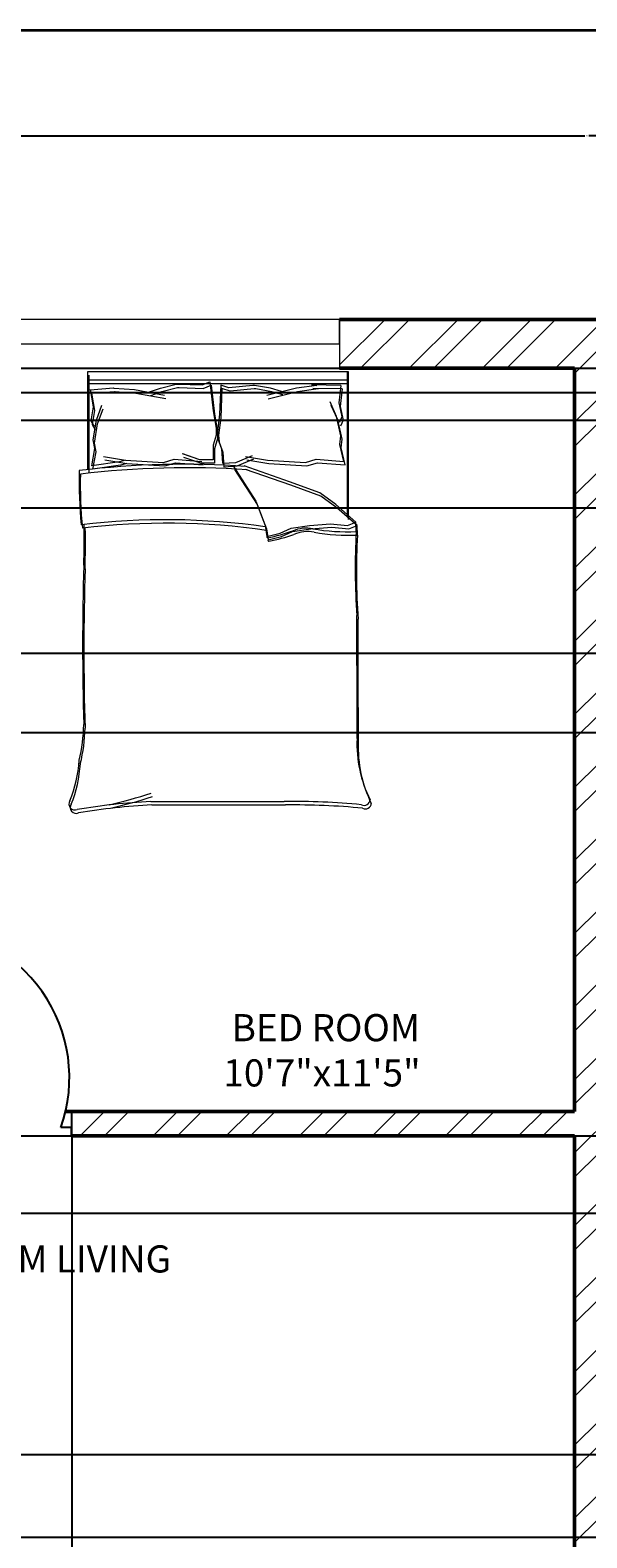
# Model space of a CAD drawing. Units: inches. Extents: x 2310 to 2937, y 1113 to 2410.
# Tile 19 of 23: x 2507 to 2609, y 2132 to 2410. Entities that reach past the tile are written whole.
import ezdxf

# ---------------------------------------------------------------- set-up
doc = ezdxf.new("R2010")
doc.units = ezdxf.units.IN
for name, color, linetype, lineweight in [('A-ANNO-DIMS', 2, 'Continuous', 18), ('A-ANNO-TTLB', 7, 'Continuous', 35), ('A-AREA-IDEN', 7, 'Continuous', 18), ('A-DOOR', 31, 'Continuous', 25), ('A-FURN', 8, 'Continuous', 18), ('A-GLAZ', 191, 'Continuous', 20), ('A-WALL', 7, 'Continuous', 50), ('A-WALL-PATT', 85, 'Continuous', 13)]:
    doc.layers.add(name, color=color, linetype=linetype, lineweight=lineweight)
doc.styles.get("Standard").update_dxf_attribs({"font": 'arial.ttf'})
doc.dimstyles.get("Standard").update_dxf_attribs({"dimtxt": 0.18, "dimasz": 0.18, "dimexe": 0.18, "dimexo": 0.0625, "dimgap": 0.09, "dimtad": 0, "dimtih": 1, "dimtoh": 1, "dimdec": 4, "dimzin": 0, "dimdsep": 46, "dimtxsty": 'Standard', "dimcen": 0.09, "dimadec": 0, "dimazin": 0, "dimtfac": 1, "dimtdec": 4, "dimtofl": 0, "dimtmove": 0, "dimatfit": 3, "dimfxl": 1, "dimtolj": 1, "dimtzin": 0, "dimarcsym": 0})

# ---------------------------------------------------------------- blocks, each defined once
blk = doc.blocks.new('BED-DOUBLE')
for p, q in [((3.56, 63.44), (3.56, 81.55)), ((3.56, 63.44), (3.56, 81.55)), ((3.56, 81.55), (51.58, 81.55)), ((3.79, 62.8), (3.79, 80.91)), ((3.79, 62.8), (3.79, 80.91)), ((51.35, 81.55), (51.35, 54.94)), ((51.35, 81.55), (51.35, 54.94)), ((51.58, 81.55), (51.58, 80.91)), ((51.58, 80.91), (51.58, 54.3)), ((51.58, 80.91), (51.58, 54.3)), ((3.56, 80.01), (51.35, 80.01)), ((3.56, 80.01), (51.35, 80.01)), ((3.79, 79.38), (51.58, 79.38)), ((3.79, 79.38), (51.58, 79.38)), ((3.98, 78.21), (8.27, 78.54)), ((3.98, 78.23), (4.56, 75.05)), ((3.98, 78.23), (4.56, 75.05)), ((3.99, 78.21), (8.27, 78.54)), ((4.21, 77.57), (8.49, 77.9)), ((4.21, 77.57), (8.49, 77.9)), ((8.27, 78.54), (8.37, 78.52)), ((8.27, 78.54), (8.37, 78.52)), ((8.37, 78.52), (12.19, 78.23)), ((8.37, 78.52), (12.19, 78.23)), ((8.49, 77.9), (8.6, 77.88)), ((8.49, 77.9), (8.6, 77.88)), ((8.6, 77.88), (12.42, 77.59)), ((8.6, 77.88), (12.42, 77.59)), ((12.19, 78.23), (17.69, 77.22)), ((12.19, 78.23), (17.69, 77.22)), ((14.94, 77.8), (16.97, 78.52)), ((14.94, 77.8), (16.96, 78.52)), ((15.17, 77.16), (17.19, 77.88)), ((15.17, 77.16), (17.19, 77.88)), ((16.96, 78.52), (19.86, 79.24)), ((16.97, 78.52), (19.86, 79.24)), ((17.19, 77.88), (20.08, 78.61)), ((17.19, 77.88), (20.08, 78.61)), ((19.86, 79.24), (20.18, 79.24)), ((19.86, 79.24), (20.18, 79.24)), ((20.08, 78.61), (20.41, 78.61)), ((20.08, 78.61), (20.41, 78.61)), ((20.18, 79.24), (24.62, 79.1)), ((20.18, 79.24), (24.62, 79.1)), ((20.41, 78.61), (24.85, 78.46)), ((20.41, 78.61), (24.85, 78.46)), ((24.62, 79.1), (26.07, 79.68)), ((24.62, 79.1), (26.07, 79.68)), ((24.85, 78.46), (26.3, 79.04)), ((24.85, 78.46), (26.3, 79.04)), ((26.07, 79.68), (26.65, 74.33)), ((26.07, 79.68), (26.65, 74.33)), ((26.3, 79.04), (26.88, 73.69)), ((26.3, 79.04), (26.88, 73.69)), ((28.06, 79.06), (27.82, 73.68)), ((28.06, 79.06), (27.82, 73.68)), ((28.29, 78.42), (28.05, 73.04)), ((28.29, 78.42), (28.05, 73.04)), ((29.54, 78.57), (28.06, 79.06)), ((29.54, 78.57), (28.06, 79.06)), ((29.77, 77.93), (28.29, 78.42)), ((29.77, 77.93), (28.29, 78.42)), ((33.97, 78.99), (29.54, 78.57)), ((33.97, 78.99), (29.54, 78.57)), ((34.2, 78.35), (29.77, 77.93)), ((34.2, 78.35), (29.77, 77.93)), ((34.29, 79.01), (33.97, 78.99)), ((34.29, 79.01), (33.97, 78.99)), ((34.52, 78.37), (34.2, 78.35)), ((34.52, 78.37), (34.2, 78.35)), ((37.22, 78.47), (34.29, 79.01)), ((37.22, 78.47), (34.29, 79.01)), ((37.45, 77.83), (34.52, 78.37)), ((37.45, 77.83), (34.52, 78.37)), ((42, 78.48), (36.58, 77.13)), ((42, 78.48), (36.58, 77.13)), ((42.23, 77.84), (36.81, 76.49)), ((42.23, 77.84), (36.81, 76.49)), ((39.29, 77.87), (37.22, 78.47)), ((39.29, 77.87), (37.22, 78.47)), ((39.52, 77.24), (37.45, 77.83)), ((39.51, 77.24), (37.45, 77.83)), ((45.8, 79.01), (42, 78.48)), ((45.8, 79.01), (42, 78.48)), ((46.03, 78.37), (42.23, 77.84)), ((46.03, 78.37), (42.23, 77.84)), ((50.2, 78.99), (44.8, 79.09)), ((44.8, 79.09), (45.8, 79.01)), ((50.2, 78.99), (44.8, 79.09)), ((44.8, 79.09), (45.8, 79.01)), ((50.43, 78.35), (45.02, 78.45)), ((45.02, 78.45), (46.03, 78.37)), ((50.43, 78.35), (45.02, 78.45)), ((45.02, 78.45), (46.03, 78.37)), ((50.2, 78.99), (49.82, 75.78)), ((50.2, 78.99), (49.82, 75.78)), ((50.43, 78.35), (50.05, 75.14)), ((50.43, 78.35), (50.05, 75.14)), ((4.56, 75.05), (4.13, 72.45)), ((4.56, 75.05), (4.13, 72.45)), ((4.21, 77.59), (4.79, 74.41)), ((4.21, 77.59), (4.79, 74.41)), ((5.14, 72.59), (6.15, 75.34)), ((5.14, 72.59), (6.15, 75.34)), ((12.42, 77.59), (17.92, 76.58)), ((12.42, 77.59), (17.92, 76.58)), ((49.4, 73.29), (48.21, 75.97)), ((49.4, 73.29), (48.21, 75.97)), ((49.62, 72.65), (48.44, 75.33)), ((49.62, 72.65), (48.44, 75.33)), ((49.82, 75.78), (50.42, 73.21)), ((49.82, 75.78), (50.41, 73.21)), ((50.05, 75.14), (50.64, 72.57)), ((50.05, 75.14), (50.64, 72.57)), ((4.13, 72.45), (4.7, 71.44)), ((4.13, 72.45), (4.7, 71.44)), ((4.79, 74.41), (4.35, 71.81)), ((4.79, 74.41), (4.35, 71.81)), ((4.56, 68.98), (5.14, 72.59)), ((4.56, 68.98), (5.14, 72.59)), ((5.37, 71.95), (6.38, 74.7)), ((5.37, 71.95), (6.38, 74.7)), ((26.65, 74.33), (27.23, 71.15)), ((26.65, 74.33), (27.23, 71.15)), ((26.88, 73.69), (27.45, 70.51)), ((26.88, 73.69), (27.45, 70.51)), ((27.82, 73.68), (27.44, 70.47)), ((27.82, 73.68), (27.44, 70.47)), ((28.05, 73.04), (27.67, 69.83)), ((28.05, 73.04), (27.67, 69.83)), ((50.2, 69.72), (49.4, 73.29)), ((50.2, 69.72), (49.4, 73.29)), ((50.43, 69.08), (49.62, 72.65)), ((50.43, 69.08), (49.62, 72.65)), ((50.42, 73.21), (49.9, 72.16)), ((50.41, 73.21), (49.9, 72.16)), ((50.64, 72.57), (50.13, 71.52)), ((50.64, 72.57), (50.13, 71.52)), ((4.35, 71.81), (4.93, 70.8)), ((4.35, 71.81), (4.93, 70.8)), ((4.79, 68.34), (5.37, 71.95)), ((4.79, 68.34), (5.37, 71.95)), ((27.23, 69.85), (26.65, 67.97)), ((27.23, 69.85), (26.65, 67.97)), ((27.23, 71.15), (27.23, 69.85)), ((27.23, 71.15), (27.23, 69.85)), ((27.44, 70.47), (27.52, 69.17)), ((27.44, 70.47), (27.52, 69.17)), ((27.45, 70.51), (27.45, 69.21)), ((27.45, 70.51), (27.45, 69.21)), ((27.67, 69.83), (27.75, 68.53)), ((27.67, 69.83), (27.75, 68.53)), ((50.01, 68.11), (50.2, 69.72)), ((50.01, 68.11), (50.2, 69.72)), ((4.27, 64.21), (4.85, 67.39)), ((4.27, 64.21), (4.85, 67.39)), ((4.5, 63.57), (5.08, 66.75)), ((4.5, 63.57), (5.08, 66.75)), ((4.85, 67.39), (4.56, 68.98)), ((4.85, 67.39), (4.56, 68.98)), ((5.08, 66.75), (4.79, 68.34)), ((5.08, 66.75), (4.79, 68.34)), ((26.65, 67.97), (26.65, 65.29)), ((26.65, 67.97), (26.65, 65.29)), ((27.45, 69.21), (26.88, 67.33)), ((27.45, 69.21), (26.88, 67.33)), ((26.88, 67.33), (26.88, 64.65)), ((26.88, 67.33), (26.88, 64.65)), ((27.52, 69.17), (28.22, 67.33)), ((27.52, 69.17), (28.22, 67.33)), ((27.75, 68.53), (28.45, 66.69)), ((27.75, 68.53), (28.44, 66.69)), ((28.22, 67.33), (28.38, 64.66)), ((28.22, 67.33), (28.38, 64.66)), ((50.78, 64.98), (50.01, 68.11)), ((50.78, 64.98), (50.01, 68.11)), ((50.24, 67.48), (50.43, 69.08)), ((50.24, 67.48), (50.43, 69.08)), ((51.01, 64.34), (50.24, 67.48)), ((51.01, 64.34), (50.24, 67.48)), ((9.37, 64.93), (4.27, 64.21)), ((9.37, 64.93), (4.27, 64.21)), ((9.6, 64.29), (4.5, 63.57)), ((9.6, 64.29), (4.5, 63.57)), ((6.47, 65.92), (10.5, 65.25)), ((6.47, 65.92), (10.5, 65.25)), ((6.7, 65.28), (10.73, 64.61)), ((6.7, 65.28), (10.73, 64.61)), ((10.5, 65.25), (9.37, 64.93)), ((10.5, 65.25), (9.37, 64.93)), ((10.73, 64.61), (9.6, 64.29)), ((10.73, 64.61), (9.6, 64.29)), ((10.5, 65.25), (17.51, 64.82)), ((10.5, 65.25), (17.51, 64.82)), ((10.73, 64.61), (17.74, 64.18)), ((10.73, 64.61), (17.74, 64.18)), ((17.51, 64.82), (19.47, 65.38)), ((17.51, 64.82), (19.47, 65.38)), ((17.74, 64.18), (19.7, 64.74)), ((17.74, 64.18), (19.7, 64.74)), ((19.47, 65.38), (24.6, 64.98)), ((19.47, 65.38), (24.6, 64.98)), ((19.7, 64.74), (24.83, 64.34)), ((19.7, 64.74), (24.83, 64.34)), ((24.19, 65.29), (21.04, 66.38)), ((24.19, 65.29), (21.05, 66.38)), ((24.42, 64.65), (21.27, 65.74)), ((24.42, 64.65), (21.27, 65.74)), ((26.65, 65.29), (24.19, 65.29)), ((26.65, 65.29), (24.19, 65.29)), ((26.88, 64.65), (24.42, 64.65)), ((26.88, 64.65), (24.42, 64.65)), ((28.38, 64.66), (30.84, 64.81)), ((28.38, 64.66), (30.84, 64.81)), ((28.44, 66.69), (28.61, 64.02)), ((28.45, 66.69), (28.61, 64.02)), ((28.61, 64.02), (31.07, 64.17)), ((28.61, 64.02), (31.06, 64.17)), ((30.35, 64.17), (34.54, 57.67)), ((30.35, 64.17), (34.54, 57.67)), ((30.84, 64.81), (33.91, 66.09)), ((30.84, 64.81), (33.91, 66.09)), ((31.06, 64.17), (34.14, 65.45)), ((31.07, 64.17), (34.14, 65.45)), ((40.73, 61.23), (32.39, 64.17)), ((40.73, 61.23), (32.39, 64.17)), ((32.65, 65.92), (36.68, 65.25)), ((32.65, 65.92), (36.68, 65.25)), ((32.88, 65.28), (36.91, 64.61)), ((32.88, 65.28), (36.91, 64.61)), ((36.68, 65.25), (43.69, 64.82)), ((36.68, 65.25), (43.69, 64.82)), ((36.91, 64.61), (43.92, 64.18)), ((36.91, 64.61), (43.92, 64.18)), ((43.69, 64.82), (45.65, 65.38)), ((43.69, 64.82), (45.65, 65.38)), ((43.92, 64.18), (45.88, 64.74)), ((43.92, 64.18), (45.88, 64.74)), ((45.65, 65.38), (50.78, 64.98)), ((45.65, 65.38), (50.78, 64.98)), ((45.88, 64.74), (51.01, 64.34)), ((45.88, 64.74), (51.01, 64.34)), ((30.57, 63.53), (34.76, 57.03)), ((30.57, 63.53), (34.76, 57.03)), ((40.96, 60.59), (32.62, 63.53)), ((40.96, 60.59), (32.62, 63.53)), ((46.31, 59.22), (40.73, 61.23)), ((46.31, 59.22), (40.73, 61.23)), ((46.53, 58.58), (40.96, 60.59)), ((46.53, 58.58), (40.96, 60.59)), ((49.25, 57.05), (46.31, 59.22)), ((49.25, 57.05), (46.31, 59.22)), ((49.48, 56.41), (46.53, 58.58)), ((49.48, 56.41), (46.53, 58.58)), ((34.54, 57.67), (36.24, 53.18)), ((34.54, 57.67), (36.24, 53.18)), ((34.76, 57.03), (36.47, 52.54)), ((34.76, 57.03), (36.47, 52.54)), ((52.95, 53.8), (49.25, 57.05)), ((52.95, 53.8), (49.25, 57.05)), ((53.18, 53.16), (49.48, 56.41)), ((53.18, 53.16), (49.48, 56.41)), ((36.24, 53.18), (36.55, 51.17)), ((36.24, 53.18), (36.55, 51.17)), ((41.04, 52.72), (44.45, 53.18)), ((41.04, 52.72), (44.45, 53.18)), ((44.45, 53.18), (48.32, 53.49)), ((44.45, 53.18), (48.32, 53.49)), ((44.68, 52.54), (48.55, 52.85)), ((44.68, 52.54), (48.55, 52.85)), ((48.32, 53.49), (51.42, 53.18)), ((48.32, 53.49), (51.42, 53.18)), ((48.55, 52.85), (51.65, 52.54)), ((48.55, 52.85), (51.65, 52.54)), ((51.42, 53.18), (52.95, 53.8)), ((51.42, 53.18), (52.95, 53.8)), ((51.65, 52.54), (53.18, 53.16)), ((51.65, 52.54), (53.18, 53.16)), ((53.03, 52.06), (52.95, 53.8, 3.87)), ((53.03, 52.06), (52.95, 53.8, 3.87)), ((53.26, 51.42), (53.18, 53.16, 3.87)), ((53.26, 51.42), (53.18, 53.16, 3.87)), ((36.47, 52.54), (36.78, 50.53)), ((36.47, 52.54), (36.78, 50.53)), ((36.55, 51.17), (39.03, 51.79)), ((36.55, 51.17), (39.03, 51.79)), ((36.78, 50.53), (39.26, 51.15)), ((36.78, 50.53), (39.26, 51.15)), ((39.03, 51.79), (41.04, 52.72)), ((39.03, 51.79), (41.04, 52.72)), ((39.26, 51.15), (41.27, 52.08)), ((39.26, 51.15), (41.27, 52.08)), ((41.27, 52.08), (44.68, 52.54)), ((41.27, 52.08), (44.68, 52.54)), ((15.15, 2.3), (39.76, 2.3)), ((15.15, 2.3), (39.76, 2.3)), ((15.38, 1.66), (39.99, 1.66)), ((15.38, 1.66), (39.99, 1.66))]:
    blk.add_line(p, q)
for centre, radius, start, end in [((21.45, -100.5), 164.97, 86.0865, 96.7821), ((21.45, -100.5), 164.97, 86.0865, 96.7821), ((85.25, 61.45), 83.31, 178.7218, 185.604), ((85.25, 61.45), 83.31, 178.7218, 185.604), ((85.48, 60.81), 83.31, 178.7218, 185.604), ((85.48, 60.81), 83.31, 178.7218, 185.604), ((21.67, -101.14), 164.97, 86.0865, 96.7821), ((21.67, -101.14), 164.97, 86.0865, 96.7821), ((17.84, -74.77), 129.02, 81.7845, 96.9006), ((17.84, -74.77), 129.02, 81.7845, 96.9006), ((18.07, -75.41), 129.02, 81.7845, 96.9006), ((18.07, -75.41), 129.02, 81.7845, 96.9006), ((-167.22, 50.37), 170.11, 358.4762, 1.0082), ((-167.22, 50.37), 170.11, 358.4762, 1.0082), ((-166.99, 49.74), 170.11, 358.4762, 1.0082), ((-166.99, 49.74), 170.11, 358.4762, 1.0082), ((36.72, 51.11), 0.185, 160.2464, 271.1377), ((36.72, 51.11), 0.185, 160.2464, 271.1377), ((31.24, 80.07), 29.65, 280.6617, 289.8806), ((31.24, 80.07), 29.65, 280.6617, 289.8806), ((36.95, 50.47), 0.185, 160.2464, 271.1377), ((36.95, 50.47), 0.185, 160.2464, 271.1377), ((31.47, 79.43), 29.65, 280.6617, 289.8806), ((31.47, 79.43), 29.65, 280.6617, 289.8806), ((43.83, 46.48), 6.22, 78.6608, 113.7384), ((43.83, 46.48), 6.22, 78.6608, 113.7384), ((44.06, 45.84), 6.22, 78.6608, 113.7384), ((44.06, 45.84), 6.22, 78.6608, 113.7384), ((51.41, 88.2), 36.18, 259.8763, 272.5657), ((51.41, 88.2), 36.18, 259.8763, 272.5657), ((51.64, 87.57), 36.18, 259.8763, 272.5657), ((51.64, 87.57), 36.18, 259.8763, 272.5657), ((182.35, 45.23), 129.5, 176.9791, 183.8365), ((182.35, 45.23), 129.5, 176.9791, 183.8365), ((182.58, 44.59), 129.5, 176.9791, 183.8365), ((182.58, 44.59), 129.5, 176.9791, 183.8365), ((484.91, 30.93), 482.31, 178.2277, 181.7185), ((484.91, 30.93), 482.31, 178.2277, 181.7185), ((485.14, 30.3), 482.31, 178.2277, 181.7185), ((485.14, 30.3), 482.31, 178.2277, 181.7185), ((-4508.66, 13.73), 4561.86, 0.00217, 0.28689), ((-4508.66, 13.73), 4561.86, 0.00217, 0.28689), ((-4508.43, 13.09), 4561.86, 0.00217, 0.28689), ((-4508.43, 13.09), 4561.86, 0.00217, 0.28689), ((-26.81, 17.03), 29.63, 346.0648, 358.9113), ((-26.81, 17.03), 29.63, 346.0648, 358.9113), ((-26.58, 16.39), 29.63, 346.0648, 358.9113), ((-26.58, 16.39), 29.63, 346.0648, 358.9113), ((76.24, 12.88), 23.07, 177.4714, 206.4681), ((76.24, 12.88), 23.07, 177.4714, 206.4681), ((76.47, 12.24), 23.07, 177.4714, 206.4681), ((76.47, 12.24), 23.07, 177.4714, 206.4681), ((-21.57, 11.27), 23.56, 337.9751, 356.652), ((-21.57, 11.27), 23.56, 337.9751, 356.652), ((-21.34, 10.63), 23.56, 337.9751, 356.652), ((-21.34, 10.63), 23.56, 337.9751, 356.652), ((-17.14, 105.26), 106.46, 283.3832, 287.7053), ((-17.14, 105.26), 106.46, 283.3832, 287.7053), ((-16.91, 104.62), 106.46, 283.3832, 287.7053), ((-16.91, 104.62), 106.46, 283.3832, 287.7053), ((1.17, 1.83), 1.09, 146.1736, 293.4781), ((1.17, 1.83), 1.09, 146.1736, 293.4781), ((1.4, 1.19), 1.09, 146.1736, 293.4781), ((1.4, 1.19), 1.09, 146.1736, 293.4781), ((21.51, -119.29), 121.76, 92.9958, 99.4091), ((21.51, -119.29), 121.76, 92.9958, 99.4091), ((21.74, -119.93), 121.76, 92.9958, 99.4091), ((21.74, -119.93), 121.76, 92.9958, 99.4091), ((41.24, -130.73), 133.04, 84.4998, 90.6351), ((41.24, -130.73), 133.04, 84.4998, 90.6351), ((41.47, -131.37), 133.04, 84.4998, 90.6351), ((41.47, -131.37), 133.04, 84.4998, 90.6351), ((54.5, 2.68), 1.1, 242.6588, 356.02), ((54.5, 2.68), 1.1, 242.6588, 356.02), ((54.72, 2.04), 1.1, 242.6588, 356.02), ((54.72, 2.04), 1.1, 242.6588, 356.02)]:
    blk.add_arc(centre, radius, start, end)
blk = doc.blocks.new('WIN-60IN-HEAD')
for p, q in [((0, 0), (0, 9)), ((0, 9), (0, 4.5)), ((60, 9), (0, 9)), ((60, 4.5), (60, 9)), ((60, 9), (60, 0)), ((0, 4.5), (60, 4.5)), ((0, 0), (60, 0))]:
    blk.add_line(p, q)
blk = doc.blocks.new('*D39')
at = {"layer": 'A-ANNO-DIMS', "color": 0, "lineweight": -2, "transparency": 16777216}
for p, q in [((2394.49, 2356.58), (2394.49, 2390.54)), ((2394.67, 2390.36), (2608.84, 2390.36)), ((2823.81, 2390.36), (2609.63, 2390.36)), ((2823.99, 2356.58), (2823.99, 2390.54))]:
    blk.add_line(p, q, dxfattribs=at)
at = {"layer": 'A-ANNO-DIMS', "color": 0, "transparency": 16777216}
for points in [[(2394.67, 2390.39), (2394.67, 2390.33), (2394.49, 2390.36)], [(2823.81, 2390.39), (2823.81, 2390.33), (2823.99, 2390.36)]]:
    blk.add_solid(points, dxfattribs=at)
at = {"layer": 'Defpoints', "color": 0, "transparency": 16777216}
for p in [(2823.99, 2390.36), (2394.49, 2356.51), (2823.99, 2356.51)]:
    blk.add_point(p, dxfattribs=at)
at = {"layer": 'A-ANNO-DIMS', "color": 0, "transparency": 16777216, "insert": (2609.24, 2390.36), "char_height": 0.18, "attachment_point": 5}
blk.add_mtext('\\A1;429.5', dxfattribs=at)
blk = doc.blocks.new('*D52')
at = {"layer": 'A-ANNO-DIMS', "color": 0, "lineweight": -2, "transparency": 16777216}
for p, q in [((2403.55, 2347.51), (2858.02, 2347.51)), ((2857.84, 2347.33), (2857.84, 2342.9)), ((2857.84, 2338.1), (2857.84, 2342.54)), ((2403.55, 2337.92), (2858.02, 2337.92))]:
    blk.add_line(p, q, dxfattribs=at)
at = {"layer": 'A-ANNO-DIMS', "color": 0, "transparency": 16777216}
for points in [[(2857.81, 2347.33), (2857.87, 2347.33), (2857.84, 2347.51)], [(2857.81, 2338.1), (2857.87, 2338.1), (2857.84, 2337.92)]]:
    blk.add_solid(points, dxfattribs=at)
at = {"layer": 'Defpoints', "color": 0, "transparency": 16777216}
for p in [(2403.49, 2347.51), (2403.49, 2337.92), (2857.84, 2337.92)]:
    blk.add_point(p, dxfattribs=at)
at = {"layer": 'A-ANNO-DIMS', "color": 0, "transparency": 16777216, "insert": (2857.84, 2342.72), "char_height": 0.18, "attachment_point": 5}
blk.add_mtext('\\A1;9.59', dxfattribs=at)
blk = doc.blocks.new('*D53')
at = {"layer": 'A-ANNO-DIMS', "color": 0, "lineweight": -2, "transparency": 16777216}
for p, q in [((2403.55, 2295.01), (2858.02, 2295.01)), ((2857.84, 2294.83), (2857.84, 2287.87)), ((2857.84, 2280.55), (2857.84, 2287.51)), ((2403.55, 2280.37), (2858.02, 2280.37))]:
    blk.add_line(p, q, dxfattribs=at)
at = {"layer": 'A-ANNO-DIMS', "color": 0, "transparency": 16777216}
for points in [[(2857.81, 2294.83), (2857.87, 2294.83), (2857.84, 2295.01)], [(2857.81, 2280.55), (2857.87, 2280.55), (2857.84, 2280.37)]]:
    blk.add_solid(points, dxfattribs=at)
at = {"layer": 'Defpoints', "color": 0, "transparency": 16777216}
for p in [(2403.49, 2295.01), (2403.49, 2280.37), (2857.84, 2280.37)]:
    blk.add_point(p, dxfattribs=at)
at = {"layer": 'A-ANNO-DIMS', "color": 0, "transparency": 16777216, "insert": (2857.84, 2287.69), "char_height": 0.18, "attachment_point": 5}
blk.add_mtext('\\A1;14.644', dxfattribs=at)
blk = doc.blocks.new('*D54')
at = {"layer": 'A-ANNO-DIMS', "color": 0, "lineweight": -2, "transparency": 16777216}
for p, q in [((2403.55, 2206.01), (2858.02, 2206.01)), ((2857.84, 2205.83), (2857.84, 2199.07)), ((2857.84, 2191.94), (2857.84, 2198.7)), ((2403.55, 2191.76), (2858.02, 2191.76))]:
    blk.add_line(p, q, dxfattribs=at)
at = {"layer": 'A-ANNO-DIMS', "color": 0, "transparency": 16777216}
for points in [[(2857.81, 2205.83), (2857.87, 2205.83), (2857.84, 2206.01)], [(2857.81, 2191.94), (2857.87, 2191.94), (2857.84, 2191.76)]]:
    blk.add_solid(points, dxfattribs=at)
at = {"layer": 'Defpoints', "color": 0, "transparency": 16777216}
for p in [(2403.49, 2206.01), (2403.49, 2191.76), (2857.84, 2191.76)]:
    blk.add_point(p, dxfattribs=at)
at = {"layer": 'A-ANNO-DIMS', "color": 0, "transparency": 16777216, "insert": (2857.84, 2198.89), "char_height": 0.18, "attachment_point": 5}
blk.add_mtext('\\A1;14.255', dxfattribs=at)
blk = doc.blocks.new('*D59')
at = {"layer": 'A-ANNO-DIMS', "color": 0, "lineweight": -2, "transparency": 16777216}
for p, q in [((2480.05, 2343.04), (2858.02, 2343.04)), ((2857.84, 2342.86), (2857.84, 2332.58)), ((2857.84, 2321.94), (2857.84, 2332.22)), ((2480.05, 2321.76), (2858.02, 2321.76))]:
    blk.add_line(p, q, dxfattribs=at)
at = {"layer": 'A-ANNO-DIMS', "color": 0, "transparency": 16777216}
for points in [[(2857.81, 2342.86), (2857.87, 2342.86), (2857.84, 2343.04)], [(2857.81, 2321.94), (2857.87, 2321.94), (2857.84, 2321.76)]]:
    blk.add_solid(points, dxfattribs=at)
at = {"layer": 'Defpoints', "color": 0, "transparency": 16777216}
for p in [(2479.99, 2343.04), (2857.84, 2343.04), (2479.99, 2321.76)]:
    blk.add_point(p, dxfattribs=at)
at = {"layer": 'A-ANNO-DIMS', "color": 0, "transparency": 16777216, "insert": (2857.84, 2332.4), "char_height": 0.18, "attachment_point": 5}
blk.add_mtext('\\A1;21.28', dxfattribs=at)
blk = doc.blocks.new('*D61')
at = {"layer": 'A-ANNO-DIMS', "color": 0, "lineweight": -2, "transparency": 16777216}
for p, q in [((2484.33, 2205.95), (2484.33, 1649.5)), ((2514.27, 2205.95), (2514.27, 1649.5)), ((2484.51, 1649.68), (2498.9, 1649.68)), ((2514.09, 1649.68), (2499.69, 1649.68))]:
    blk.add_line(p, q, dxfattribs=at)
at = {"layer": 'A-ANNO-DIMS', "color": 0, "transparency": 16777216}
for points in [[(2484.51, 1649.71), (2484.51, 1649.65), (2484.33, 1649.68)], [(2514.09, 1649.71), (2514.09, 1649.65), (2514.27, 1649.68)]]:
    blk.add_solid(points, dxfattribs=at)
at = {"layer": 'Defpoints', "color": 0, "transparency": 16777216}
for p in [(2484.33, 2206.01), (2514.27, 2206.01), (2514.27, 1649.68)]:
    blk.add_point(p, dxfattribs=at)
at = {"layer": 'A-ANNO-DIMS', "color": 0, "transparency": 16777216, "insert": (2499.3, 1649.68), "char_height": 0.18, "attachment_point": 5}
blk.add_mtext('\\A1;29.94', dxfattribs=at)
blk = doc.blocks.new('*D70')
at = {"layer": 'A-ANNO-DIMS', "color": 0, "lineweight": -2, "transparency": 16777216}
for p, q in [((2475.96, 2147.28), (2858.02, 2147.28)), ((2857.84, 2147.1), (2857.84, 2139.83)), ((2857.84, 2132.2), (2857.84, 2139.47)), ((2475.96, 2132.02), (2858.02, 2132.02))]:
    blk.add_line(p, q, dxfattribs=at)
at = {"layer": 'A-ANNO-DIMS', "color": 0, "transparency": 16777216}
for points in [[(2857.81, 2147.1), (2857.87, 2147.1), (2857.84, 2147.28)], [(2857.81, 2132.2), (2857.87, 2132.2), (2857.84, 2132.02)]]:
    blk.add_solid(points, dxfattribs=at)
at = {"layer": 'Defpoints', "color": 0, "transparency": 16777216}
for p in [(2475.89, 2147.28), (2857.84, 2147.28), (2475.89, 2132.02)]:
    blk.add_point(p, dxfattribs=at)
at = {"layer": 'A-ANNO-DIMS', "color": 0, "transparency": 16777216, "insert": (2857.84, 2139.65), "char_height": 0.18, "attachment_point": 5}
blk.add_mtext('\\A1;15.257', dxfattribs=at)

msp = doc.modelspace()

# ---------------------------------------------------------------- hatches: boundary and pattern name
at = {"layer": 'A-WALL-PATT'}
h = msp.add_hatch(dxfattribs=at)
h.set_pattern_fill('ANSI32', color=256)
h.paths.add_polyline_path([(2639.1394, 2356.5139), (2563.662, 2356.5139), (2563.662, 2347.5139), (2606.9859, 2347.5139), (2606.9859, 2210.5139), (2514.2692, 2210.5139), (2514.2692, 2206.0139), (2606.9859, 2206.0139), (2606.9859, 2098.0139), (2602.689, 2098.0139), (2602.689, 2093.5139), (2615.5262, 2093.5139), (2615.5262, 2095.7639), (2615.5262, 2098.0139), (2611.4859, 2098.0139), (2611.4859, 2206.0139), (2703.9391, 2206.0139), (2703.9391, 2208.2639), (2703.9391, 2210.5139), (2611.4859, 2210.5139), (2611.4859, 2347.5139), (2639.1394, 2347.5139)])
h.paths.add_polyline_path([(2823.9859, 2356.5139), (2699.1394, 2356.5139), (2699.1394, 2347.5139), (2738.4859, 2347.5139), (2738.4859, 2343.9266), (2742.9859, 2343.9266), (2742.9859, 2347.5139), (2814.9859, 2347.5139), (2814.9859, 2336.76), (2823.9859, 2336.76)])
h.paths.add_polyline_path([(2823.9859, 2312.76), (2814.9859, 2312.76), (2814.9859, 2299.5139), (2742.9859, 2299.5139), (2742.9859, 2323.0159), (2740.7359, 2323.0159), (2738.4859, 2323.0159), (2738.4859, 2210.5139), (2734.5483, 2210.5139), (2734.5483, 2206.0139), (2746.8769, 2206.0139), (2746.8769, 2208.2639), (2746.8769, 2210.5139), (2742.9859, 2210.5139), (2742.9859, 2295.0139), (2814.9859, 2295.0139), (2814.9859, 2269.8977), (2823.9859, 2269.8977)])
h.paths.add_polyline_path([(2823.9859, 2210.5139), (2823.9859, 2233.8977), (2819.4859, 2233.8977), (2814.9859, 2233.8977), (2814.9859, 2210.5139), (2769.9745, 2210.5139), (2769.9745, 2206.0139), (2814.9859, 2206.0139), (2814.9859, 2178.3027), (2823.9859, 2178.3027)])
h.paths.add_polyline_path([(2823.9859, 2118.3027), (2819.4859, 2118.3027), (2814.9859, 2118.3027), (2814.9859, 2098.0139), (2647.0333, 2098.0139), (2647.0333, 2093.5139), (2814.9859, 2093.5139), (2814.9859, 1999.5139), (2650.6052, 1999.5139), (2650.6052, 1995.0139), (2814.9859, 1995.0139), (2814.9859, 1969.9784), (2823.9859, 1969.9784)])
h.paths.add_polyline_path([(2403.4859, 2093.5139), (2569.9888, 2093.5139), (2569.9888, 2095.7639), (2569.9888, 2098.0139), (2403.4859, 2098.0139), (2403.4859, 2131.7587), (2394.4859, 2131.7587), (2394.4859, 1967.522), (2403.4859, 1967.522), (2403.4859, 1995.0139), (2569.8903, 1995.0139), (2569.8903, 1997.2639), (2569.8903, 1999.5139), (2403.4859, 1999.5139)])
h.paths.add_polyline_path([(2503.662, 2356.5139), (2394.4859, 2356.5139), (2394.4859, 2337.9231), (2398.9859, 2337.9231), (2403.4859, 2337.9231), (2403.4859, 2347.5139), (2475.4859, 2347.5139), (2475.4859, 2343.0384), (2479.9859, 2343.0384), (2479.9859, 2347.5139), (2503.662, 2347.5139)])
h.paths.add_polyline_path([(2498.3065, 1745.5139), (2479.9859, 1745.5139), (2479.9859, 1749.1663), (2477.7359, 1749.1663), (2475.4859, 1749.1663), (2475.4859, 1745.5139), (2403.4859, 1745.5139), (2403.4859, 1753.6409), (2398.9859, 1753.6409), (2394.4859, 1753.6409), (2394.4859, 1736.5139), (2498.3065, 1736.5139), (2498.3065, 1741.0139)])
h.paths.add_polyline_path([(2479.9859, 1882.5139), (2483.9367, 1882.5139), (2483.9367, 1887.0139), (2471.5501, 1887.0139), (2471.5501, 1885.1969), (2471.5501, 1882.5139), (2475.4859, 1882.5139), (2475.4859, 1798.0139), (2403.4859, 1798.0139), (2403.4859, 1828.0433), (2402.2852, 1828.0433), (2394.4859, 1828.0433), (2394.4859, 1777.6409), (2403.4859, 1777.6409), (2403.4859, 1793.5139), (2475.4859, 1793.5139), (2475.4859, 1769.1696), (2479.9859, 1769.1696)])
h.paths.add_polyline_path([(2403.4859, 1907.522), (2398.9859, 1907.522), (2394.4859, 1907.522), (2394.4859, 1864.0433), (2403.4859, 1864.0433), (2403.4859, 1882.5139), (2448.9325, 1882.5139), (2448.9325, 1884.7639), (2448.9325, 1887.0139), (2403.4859, 1887.0139)])
h.paths.add_polyline_path([(2702.2061, 1887.0139), (2611.4859, 1887.0139), (2611.4859, 1995.0139), (2615.6132, 1995.0139), (2615.6132, 1999.5139), (2602.4798, 1999.5139), (2602.4798, 1997.2639), (2602.4798, 1995.0139), (2606.9859, 1995.0139), (2606.9859, 1887.0139), (2516.2443, 1887.0139), (2516.2443, 1884.7639), (2516.2443, 1882.5139), (2606.9859, 1882.5139), (2606.9859, 1745.5139), (2558.3065, 1745.5139), (2558.3065, 1736.5139), (2638.8921, 1736.5139), (2638.8921, 1741.0139), (2638.8921, 1745.5139), (2611.4859, 1745.5139), (2611.4859, 1882.5139), (2702.2061, 1882.5139)])
h.paths.add_polyline_path([(2823.9859, 1909.9784), (2819.4859, 1909.9784), (2814.9859, 1909.9784), (2814.9859, 1887.0139), (2769.144, 1887.0139), (2769.144, 1884.7639), (2769.144, 1882.5139), (2814.9859, 1882.5139), (2814.9859, 1854.1704), (2823.9859, 1854.1704)])
h.paths.add_polyline_path([(2823.9859, 1818.1704), (2819.4859, 1818.1704), (2814.9859, 1818.1704), (2814.9859, 1798.0139), (2742.9859, 1798.0139), (2742.9859, 1882.5139), (2746.805, 1882.5139), (2746.805, 1887.0139), (2733.7334, 1887.0139), (2733.7334, 1884.7639), (2733.7334, 1882.5139), (2738.4859, 1882.5139), (2738.4859, 1771.1728), (2740.7359, 1771.1728), (2742.9859, 1771.1728), (2742.9859, 1793.5139), (2814.9859, 1793.5139), (2814.9859, 1783.6684), (2823.9859, 1783.6684)])
h.paths.add_polyline_path([(2823.9859, 1759.6684), (2814.9859, 1759.6684), (2814.9859, 1745.5139), (2742.9859, 1745.5139), (2742.9859, 1748.9831), (2740.7359, 1748.9831), (2738.4859, 1748.9831), (2738.4859, 1745.5139), (2698.8921, 1745.5139), (2698.8921, 1736.5139), (2823.9859, 1736.5139)])

# ---------------------------------------------------------------- linework, layer by layer
at = {"layer": 'A-ANNO-TTLB'}
msp.add_lwpolyline([(2310.2498, 2409.8427), (2937.0534, 2409.8427), (2937.0534, 1616.036), (2310.2498, 1616.036)], close=True, dxfattribs=at)
at = {"layer": 'A-DOOR'}
for p, q in [((2514.2692, 2210.5139), (2514.2692, 2206.0139)), ((2514.2692, 2207.5183), (2512.2692, 2207.5183)), ((2514.2692, 2206.0139), (2514.2692, 2207.5183))]:
    msp.add_line(p, q, dxfattribs=at)
msp.add_arc((2486.3278, 2216.7342), 27.5298, 340.442065, 90, dxfattribs=at)
at = {"layer": 'A-WALL'}
for p, q in [((2563.662, 2356.5139), (2639.1394, 2356.5139)), ((2563.662, 2347.5139), (2606.9859, 2347.5139)), ((2606.9859, 2347.5139), (2606.9859, 2210.5139)), ((2513.1457, 2210.5139), (2606.9859, 2210.5139)), ((2514.2692, 2206.0139), (2606.9859, 2206.0139)), ((2606.9859, 2206.0139), (2606.9859, 2098.0139))]:
    msp.add_line(p, q, dxfattribs=at)

# ---------------------------------------------------------------- block references
at = {"layer": 'A-FURN'}
msp.add_blockref('BED-DOUBLE', (2513.6888, 2265.3421), dxfattribs=at)
at = {"layer": 'A-GLAZ'}
msp.add_blockref('WIN-60IN-HEAD', (2503.662, 2347.5139), dxfattribs=at)

# ---------------------------------------------------------------- texts
at = {"layer": 'A-AREA-IDEN', "char_height": 5, "attachment_point": 1}
for s, width, insert in [('    BED ROOM\\P   10\'7"x11\'5"', 188.724755, (2537.6458, 2228.4458)), ("    DINING CUM LIVING\\P          17'X9'", 158.341629, (2464.1081, 2185.8129))]:
    msp.add_mtext_dynamic_manual_height_columns(s, width=width, gutter_width=12.5, heights=[0], dxfattribs=dict(at, insert=insert))

# ---------------------------------------------------------------- dimensions: what is measured, and where the dimension line sits
at = {"layer": 'A-ANNO-DIMS'}
for base, p1, p2, override, picture, middle in [((2823.9859, 2390.3639), (2394.4859, 2356.5139), (2823.9859, 2356.5139), {"dimdec": 1, "dimlfac": 1, "dimrnd": 0, "dimzin": 0, "dimdsep": 46, "dimlunit": 2}, '*D39', (2609.2359, 2390.3639)), ((2514.2692, 1649.6807), (2484.3278, 2206.0139), (2514.2692, 2206.0139), {"dimdec": 2, "dimlfac": 1, "dimrnd": 0, "dimzin": 0, "dimdsep": 46, "dimlunit": 2}, '*D61', (2499.2985, 1649.6807))]:
    dim = msp.add_linear_dim(base=base, p1=p1, p2=p2, dimstyle='Standard', override=override, dxfattribs=at)
    dim.commit()
    dim.dimension.update_dxf_attribs({"geometry": picture, "text_midpoint": middle})
for base, p1, p2, override, picture, middle in [((2857.8359, 2337.9231), (2403.4859, 2347.5139), (2403.4859, 2337.9231), {"dimdec": 2, "dimlfac": 1, "dimrnd": 0, "dimzin": 0, "dimdsep": 46, "dimlunit": 2}, '*D52', (2857.8359, 2342.7185)), ((2857.8359, 2343.0384), (2479.9859, 2321.7598), (2479.9859, 2343.0384), {"dimdec": 2, "dimlfac": 1, "dimrnd": 0, "dimzin": 0, "dimdsep": 46, "dimlunit": 2}, '*D59', (2857.8359, 2332.3991)), ((2857.8359, 2280.3697), (2403.4859, 2295.0139), (2403.4859, 2280.3697), {"dimdec": 3, "dimlfac": 1, "dimrnd": 0, "dimzin": 0, "dimdsep": 46, "dimlunit": 2}, '*D53', (2857.8359, 2287.6918)), ((2857.8359, 2191.7587), (2403.4859, 2206.0139), (2403.4859, 2191.7587), {"dimdec": 3, "dimlfac": 1, "dimrnd": 0, "dimzin": 0, "dimdsep": 46, "dimlunit": 2}, '*D54', (2857.8359, 2198.8863)), ((2857.8359, 2147.2815), (2475.8929, 2132.0241), (2475.8929, 2147.2815), {"dimdec": 3, "dimlfac": 1, "dimrnd": 0, "dimzin": 0, "dimdsep": 46, "dimlunit": 2}, '*D70', (2857.8359, 2139.6528))]:
    dim = msp.add_linear_dim(base=base, p1=p1, p2=p2, angle=90, dimstyle='Standard', override=override, dxfattribs=at)
    dim.commit()
    dim.dimension.update_dxf_attribs({"geometry": picture, "text_midpoint": middle})

doc.saveas('drawing.dxf')
